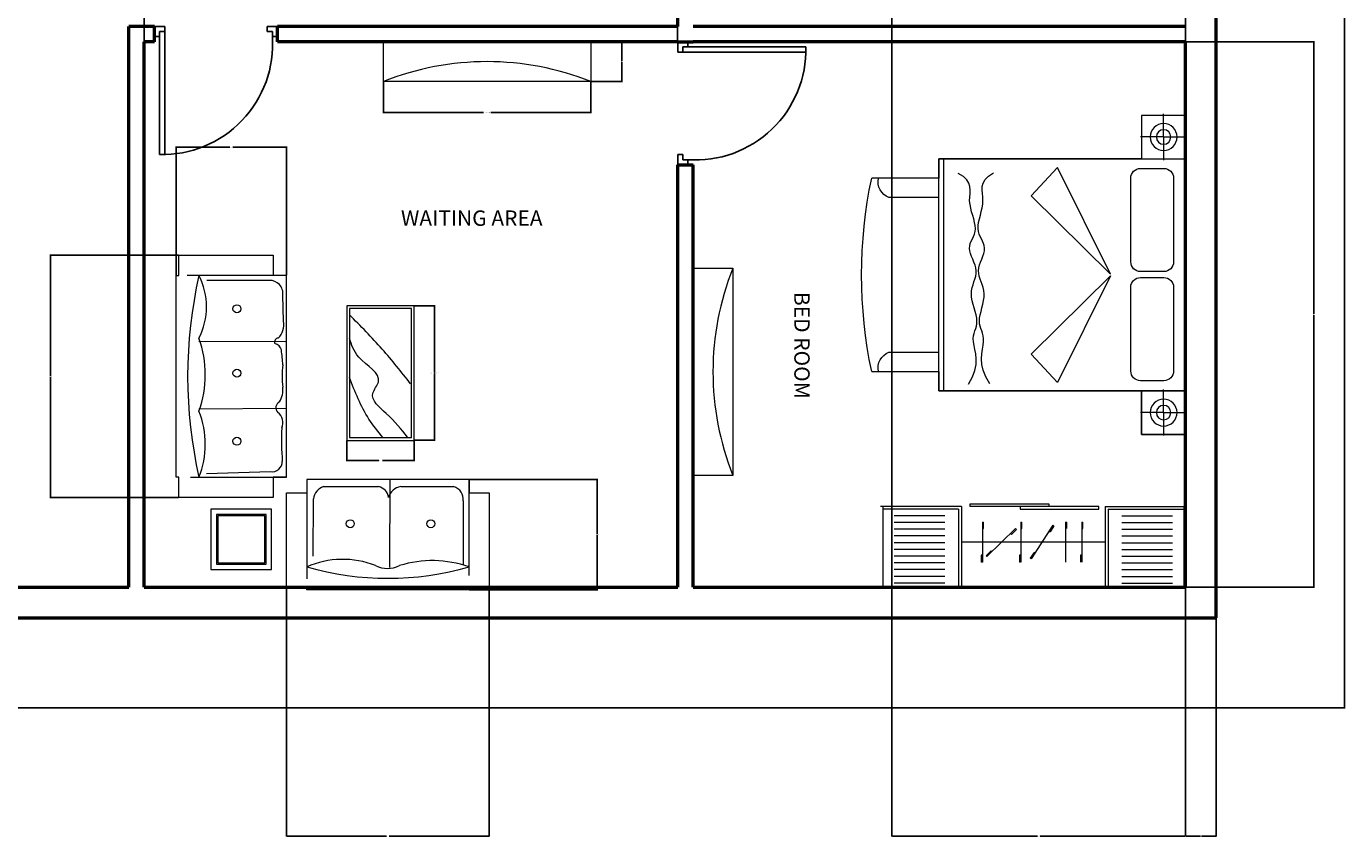
# Model space of a CAD drawing. Units: inches. Extents: x 1865 to 2541, y 1997 to 2759.
# Tile 3 of 11: x 2155 to 2541, y 1997 to 2234. Entities that reach past the tile are written whole.
import ezdxf

# ---------------------------------------------------------------- set-up
doc = ezdxf.new("R2010")
doc.units = ezdxf.units.IN
for name, color, linetype, lineweight in [('A-ANNO-DIMS', 2, 'Continuous', 18), ('A-AREA-IDEN', 4, 'Continuous', 18), ('A-FURN', 8, 'Continuous', 13), ('A-WALL', 7, 'Continuous', 50), ('BED', 42, 'Continuous', 13), ('CUPBOARD', 61, 'Continuous', 18), ('DOOR', 1, 'Continuous', 25), ('TV', 3, 'Continuous', 18)]:
    doc.layers.add(name, color=color, linetype=linetype, lineweight=lineweight)
doc.styles.get("Standard").update_dxf_attribs({"font": 'arial.ttf'})
doc.dimstyles.get("Standard").update_dxf_attribs({"dimtxt": 0.18, "dimasz": 0.18, "dimexe": 0.18, "dimexo": 0.0625, "dimgap": 0.09, "dimtad": 0, "dimtih": 1, "dimtoh": 1, "dimdec": 4, "dimzin": 0, "dimdsep": 46, "dimtxsty": 'Standard', "dimcen": 0.09, "dimadec": 0, "dimazin": 0, "dimtfac": 1, "dimtdec": 4, "dimtofl": 0, "dimtmove": 0, "dimatfit": 3, "dimfxl": 1, "dimtolj": 1, "dimtzin": 0, "dimarcsym": 0})

# ---------------------------------------------------------------- blocks, each defined once
blk = doc.blocks.new('A$C4F543DC7')
for p, q in [((0.013, 3.35, -0.169), (3.313, 3.35, -0.169)), ((0.463, 3.35, -0.169), (0.013, 3.35, -0.169)), ((0.013, 2.896, -0.169), (0.013, 3.35, -0.169)), ((0.013, 3.35, -0.169), (0.013, 2.896, -0.169)), ((0.238, 3.123, -0.439), (0.238, 3.361, -0.439)), ((0.463, 3.35, -0.169), (0.463, 0.8, -0.169)), ((2.863, 3.35, -0.169), (0.463, 3.35, -0.169)), ((0.463, 2.896, -0.169), (0.463, 3.35, -0.169)), ((2.863, 0.8, -0.169), (2.863, 3.35, -0.169)), ((2.863, 3.35, -0.169), (3.313, 3.35, -0.169)), ((2.863, 2.896, -0.169), (2.863, 3.35, -0.169)), ((3.089, 3.123, -0.439), (3.089, 3.361, -0.439)), ((3.313, 3.35, -0.169), (3.313, 2.896, -0.169)), ((3.313, 3.35, -0.169), (3.313, 2.896, -0.169)), ((1.535, 3.226, -0.169), (0.668, 3.226, -0.169)), ((2.664, 3.226, -0.169), (1.797, 3.226, -0.169)), ((0.238, 3.123, -0.439), (0, 3.123, -0.439)), ((0.238, 3.123, -0.439), (0.476, 3.123, -0.439)), ((0.238, 3.123, -0.439), (0.238, 2.885, -0.439)), ((0.568, 3.126, -0.169), (0.568, 2.884, -0.169)), ((1.635, 2.884, -0.169), (1.635, 3.126, -0.169)), ((1.697, 3.126, -0.169), (1.697, 2.884, -0.169)), ((2.764, 2.884, -0.169), (2.764, 3.126, -0.169)), ((3.089, 3.123, -0.439), (2.851, 3.123, -0.439)), ((3.089, 3.123, -0.439), (3.089, 2.885, -0.439)), ((3.089, 3.123, -0.439), (3.327, 3.123, -0.439)), ((0.463, 2.896, -0.169), (0.013, 2.896, -0.169)), ((0.013, 2.896, -0.169), (0.463, 2.896, -0.169)), ((0.463, 0.8, -0.169), (0.463, 2.896, -0.169)), ((2.863, 2.896, -0.169), (2.863, 0.8, -0.169)), ((3.313, 2.896, -0.169), (2.863, 2.896, -0.169)), ((3.313, 2.896, -0.169), (2.863, 2.896, -0.169)), ((0.668, 2.784, -0.169), (1.535, 2.784, -0.169)), ((1.797, 2.784, -0.169), (2.664, 2.784, -0.169)), ((1.653, 2.573, -0.169), (0.55, 2.025, -0.169)), ((0.841, 1.752, -0.169), (1.653, 2.573, -0.169)), ((2.481, 1.752, -0.169), (1.669, 2.573, -0.169)), ((1.669, 2.573, -0.169), (2.772, 2.025, -0.169)), ((0.55, 2.025, -0.169), (0.841, 1.752, -0.169)), ((2.772, 2.025, -0.169), (2.481, 1.752, -0.169)), ((0.537, 1.327, -0.169), (0.609, 1.284, -0.169)), ((0.609, 1.284, -0.169), (0.676, 1.257, -0.169)), ((0.676, 1.257, -0.169), (0.737, 1.243, -0.169)), ((0.737, 1.243, -0.169), (0.794, 1.239, -0.169)), ((0.794, 1.239, -0.169), (0.846, 1.242, -0.169)), ((0.846, 1.242, -0.169), (0.893, 1.249, -0.169)), ((0.893, 1.249, -0.169), (0.935, 1.256, -0.169)), ((0.935, 1.256, -0.169), (0.972, 1.261, -0.169)), ((0.972, 1.261, -0.169), (1.004, 1.262, -0.169)), ((1.004, 1.262, -0.169), (1.033, 1.258, -0.169)), ((1.033, 1.258, -0.169), (1.06, 1.251, -0.169)), ((1.06, 1.251, -0.169), (1.084, 1.242, -0.169)), ((1.084, 1.242, -0.169), (1.108, 1.234, -0.169)), ((1.108, 1.234, -0.169), (1.132, 1.226, -0.169)), ((1.25, 1.226, -0.169), (1.285, 1.235, -0.169)), ((1.285, 1.235, -0.169), (1.322, 1.244, -0.169)), ((1.322, 1.244, -0.169), (1.359, 1.253, -0.169)), ((1.359, 1.253, -0.169), (1.396, 1.261, -0.169)), ((1.396, 1.261, -0.169), (1.433, 1.266, -0.169)), ((1.433, 1.266, -0.169), (1.468, 1.268, -0.169)), ((1.468, 1.268, -0.169), (1.501, 1.264, -0.169)), ((1.501, 1.264, -0.169), (1.532, 1.257, -0.169)), ((1.532, 1.257, -0.169), (1.562, 1.247, -0.169)), ((1.562, 1.247, -0.169), (1.591, 1.237, -0.169)), ((1.591, 1.237, -0.169), (1.62, 1.226, -0.169)), ((1.765, 1.22, -0.169), (1.795, 1.23, -0.169)), ((1.795, 1.23, -0.169), (1.826, 1.242, -0.169)), ((1.826, 1.242, -0.169), (1.856, 1.253, -0.169)), ((1.856, 1.253, -0.169), (1.885, 1.263, -0.169)), ((1.885, 1.263, -0.169), (1.913, 1.27, -0.169)), ((1.913, 1.27, -0.169), (1.94, 1.272, -0.169)), ((1.94, 1.272, -0.169), (1.965, 1.269, -0.169)), ((1.965, 1.269, -0.169), (1.989, 1.262, -0.169)), ((1.989, 1.262, -0.169), (2.012, 1.251, -0.169)), ((2.012, 1.251, -0.169), (2.036, 1.239, -0.169)), ((2.036, 1.239, -0.169), (2.06, 1.227, -0.169)), ((2.279, 1.228, -0.169), (2.317, 1.238, -0.169)), ((2.317, 1.238, -0.169), (2.356, 1.246, -0.169)), ((2.356, 1.246, -0.169), (2.394, 1.253, -0.169)), ((2.394, 1.253, -0.169), (2.433, 1.255, -0.169)), ((2.433, 1.255, -0.169), (2.47, 1.253, -0.169)), ((2.47, 1.253, -0.169), (2.506, 1.249, -0.169)), ((2.506, 1.249, -0.169), (2.542, 1.246, -0.169)), ((2.542, 1.246, -0.169), (2.578, 1.248, -0.169)), ((2.578, 1.248, -0.169), (2.613, 1.257, -0.169)), ((2.613, 1.257, -0.169), (2.648, 1.277, -0.169)), ((2.648, 1.277, -0.169), (2.683, 1.312, -0.169)), ((2.683, 1.312, -0.169), (2.718, 1.364, -0.169)), ((0.533, 1.105, -0.169), (0.607, 1.146, -0.169)), ((0.607, 1.146, -0.169), (0.674, 1.171, -0.169)), ((0.674, 1.171, -0.169), (0.736, 1.183, -0.169)), ((0.736, 1.183, -0.169), (0.793, 1.185, -0.169)), ((0.793, 1.185, -0.169), (0.845, 1.18, -0.169)), ((0.845, 1.18, -0.169), (0.891, 1.172, -0.169)), ((0.891, 1.172, -0.169), (0.933, 1.163, -0.169)), ((0.933, 1.163, -0.169), (0.97, 1.156, -0.169)), ((0.97, 1.156, -0.169), (1.003, 1.155, -0.169)), ((1.003, 1.155, -0.169), (1.032, 1.158, -0.169)), ((1.032, 1.158, -0.169), (1.058, 1.164, -0.169)), ((1.058, 1.164, -0.169), (1.083, 1.172, -0.169)), ((1.083, 1.172, -0.169), (1.107, 1.18, -0.169)), ((1.107, 1.18, -0.169), (1.132, 1.187, -0.169)), ((1.132, 1.226, -0.169), (1.158, 1.22, -0.169)), ((1.132, 1.187, -0.169), (1.157, 1.192, -0.169)), ((1.157, 1.192, -0.169), (1.185, 1.193, -0.169)), ((1.158, 1.22, -0.169), (1.185, 1.218, -0.169)), ((1.185, 1.218, -0.169), (1.216, 1.22, -0.169)), ((1.185, 1.193, -0.169), (1.216, 1.19, -0.169)), ((1.216, 1.22, -0.169), (1.25, 1.226, -0.169)), ((1.216, 1.19, -0.169), (1.249, 1.183, -0.169)), ((1.249, 1.183, -0.169), (1.284, 1.173, -0.169)), ((1.284, 1.173, -0.169), (1.321, 1.163, -0.169)), ((1.321, 1.163, -0.169), (1.358, 1.152, -0.169)), ((1.358, 1.152, -0.169), (1.394, 1.143, -0.169)), ((1.394, 1.143, -0.169), (1.431, 1.137, -0.169)), ((1.431, 1.137, -0.169), (1.466, 1.135, -0.169)), ((1.466, 1.135, -0.169), (1.499, 1.137, -0.169)), ((1.499, 1.137, -0.169), (1.531, 1.143, -0.169)), ((1.531, 1.143, -0.169), (1.561, 1.152, -0.169)), ((1.561, 1.152, -0.169), (1.59, 1.162, -0.169)), ((1.59, 1.162, -0.169), (1.619, 1.172, -0.169)), ((1.619, 1.172, -0.169), (1.648, 1.18, -0.169)), ((1.62, 1.226, -0.169), (1.648, 1.217, -0.169)), ((1.648, 1.217, -0.169), (1.676, 1.211, -0.169)), ((1.648, 1.18, -0.169), (1.676, 1.185, -0.169)), ((1.676, 1.211, -0.169), (1.705, 1.209, -0.169)), ((1.676, 1.185, -0.169), (1.705, 1.186, -0.169)), ((1.705, 1.209, -0.169), (1.735, 1.212, -0.169)), ((1.705, 1.186, -0.169), (1.734, 1.182, -0.169)), ((1.734, 1.182, -0.169), (1.764, 1.173, -0.169)), ((1.735, 1.212, -0.169), (1.765, 1.22, -0.169)), ((1.764, 1.173, -0.169), (1.794, 1.162, -0.169)), ((1.794, 1.162, -0.169), (1.824, 1.149, -0.169)), ((1.824, 1.149, -0.169), (1.854, 1.137, -0.169)), ((1.854, 1.137, -0.169), (1.883, 1.126, -0.169)), ((1.883, 1.126, -0.169), (1.911, 1.119, -0.169)), ((1.911, 1.119, -0.169), (1.937, 1.115, -0.169)), ((1.937, 1.115, -0.169), (1.963, 1.118, -0.169)), ((1.963, 1.118, -0.169), (1.987, 1.124, -0.169)), ((1.987, 1.124, -0.169), (2.011, 1.134, -0.169)), ((2.011, 1.134, -0.169), (2.034, 1.145, -0.169)), ((2.034, 1.145, -0.169), (2.059, 1.157, -0.169)), ((2.059, 1.157, -0.169), (2.084, 1.167, -0.169)), ((2.06, 1.227, -0.169), (2.085, 1.216, -0.169)), ((2.084, 1.167, -0.169), (2.111, 1.174, -0.169)), ((2.085, 1.216, -0.169), (2.112, 1.208, -0.169)), ((2.111, 1.174, -0.169), (2.14, 1.177, -0.169)), ((2.112, 1.208, -0.169), (2.141, 1.204, -0.169)), ((2.14, 1.177, -0.169), (2.172, 1.175, -0.169)), ((2.141, 1.204, -0.169), (2.172, 1.205, -0.169)), ((2.172, 1.205, -0.169), (2.206, 1.21, -0.169)), ((2.172, 1.175, -0.169), (2.206, 1.169, -0.169)), ((2.206, 1.21, -0.169), (2.242, 1.218, -0.169)), ((2.206, 1.169, -0.169), (2.241, 1.16, -0.169)), ((2.241, 1.16, -0.169), (2.278, 1.149, -0.169)), ((2.242, 1.218, -0.169), (2.279, 1.228, -0.169)), ((2.278, 1.149, -0.169), (2.316, 1.138, -0.169)), ((2.316, 1.138, -0.169), (2.354, 1.128, -0.169)), ((2.354, 1.128, -0.169), (2.392, 1.121, -0.169)), ((2.392, 1.121, -0.169), (2.43, 1.117, -0.169)), ((2.43, 1.117, -0.169), (2.468, 1.118, -0.169)), ((2.468, 1.118, -0.169), (2.504, 1.121, -0.169)), ((2.504, 1.121, -0.169), (2.54, 1.123, -0.169)), ((2.54, 1.123, -0.169), (2.576, 1.12, -0.169)), ((2.576, 1.12, -0.169), (2.611, 1.109, -0.169)), ((2.611, 1.109, -0.169), (2.645, 1.088, -0.169)), ((2.645, 1.088, -0.169), (2.679, 1.052, -0.169)), ((2.679, 1.052, -0.169), (2.712, 0.999, -0.169)), ((0.463, 0.85, -0.169), (2.863, 0.85, -0.169)), ((0.463, 0.8, -0.169), (2.863, 0.8, -0.169)), ((0.663, 0.8, -0.169), (0.463, 0.8, -0.169)), ((0.663, 0.8, -0.169), (2.663, 0.8, -0.169)), ((0.663, 0.104, -0.169), (0.663, 0.8, -0.169)), ((0.663, 0.104, -0.169), (0.663, 0.8, -0.169)), ((0.863, 0.281, -0.169), (0.863, 0.8, -0.169)), ((2.463, 0.8, -0.169), (2.463, 0.281, -0.169)), ((2.863, 0.8, -0.169), (2.663, 0.8, -0.169)), ((2.663, 0.8, -0.169), (2.663, 0.104, -0.169)), ((2.663, 0.8, -0.169), (2.663, 0.104, -0.169))]:
    blk.add_line(p, q)
for centre, radius in [((0.238, 3.123, -0.439), 0.139), ((0.238, 3.123, -0.439), 0.075), ((3.089, 3.123, -0.439), 0.139), ((3.089, 3.123, -0.439), 0.075)]:
    blk.add_circle(centre, radius)
for centre, radius, start, end in [((0.668, 3.126, -0.169), 0.1, 90, 180), ((1.535, 3.126, -0.169), 0.1, 0, 90), ((1.797, 3.126, -0.169), 0.1, 90, 180), ((2.664, 3.126, -0.169), 0.1, 0, 90), ((0.668, 2.884, -0.169), 0.1, 180, 270), ((1.535, 2.884, -0.169), 0.1, 270, 0), ((1.797, 2.884, -0.169), 0.1, 180, 270), ((2.664, 2.884, -0.169), 0.1, 270, 0), ((0.699, 0.347, -0.169), 0.177, 258.2616, 338.032), ((2.627, 0.347, -0.169), 0.177, 201.968, 281.7384), ((1.663, 4.86, -0.169), 4.86, 258.1252, 281.8748), ((1.663, 4.86, -0.169), 4.86, 258.1252, 281.8748)]:
    blk.add_arc(centre, radius, start, end)
blk = doc.blocks.new('A$C34930FF8')
for p, q in [((600, 1669.3), (600, 2269.3)), ((30, 1790.9), (30, 2169.3)), ((80, 1790.9), (80, 2169.3)), ((130, 1790.9), (130, 2169.3)), ((180, 1790.9), (180, 2169.3)), ((230, 1790.9), (230, 2169.3)), ((280, 1790.9), (280, 2169.3)), ((330, 1790.9), (330, 2169.3)), ((380, 1790.9), (380, 2169.3)), ((430, 1790.9), (430, 2169.3)), ((480, 1790.9), (480, 2169.3)), ((530, 1790.9), (530, 2169.3)), ((580, 1690.9), (580, 2252.4)), ((580, 1690.9), (0, 1690.9)), ((600, 1669.3), (0, 1669.3)), ((335.4, 1666.1), (335.4, 603.1)), ((600, 1603.3), (620, 1603.3)), ((600, 1018.7), (600, 1603.3)), ((620, 1603.3), (620, 1018.7)), ((237.7, 1521.5), (185.4, 1521.5)), ((482.5, 1513), (185.4, 1513)), ((434.8, 1266.1), (227.4, 1478.9)), ((269.7, 1447.7), (233.2, 1485.2)), ((436.7, 1504.4), (482.5, 1504.4)), ((428.7, 1260.1), (392.1, 1297.6)), ((237.7, 1237.7), (185.4, 1237.7)), ((482.5, 1228.2), (185.4, 1228.2)), ((436.7, 1219.7), (482.5, 1219.7)), ((600, 1233.4), (580, 1233.4)), ((580, 1233.4), (580, 648.7)), ((600, 648.7), (600, 1233.4)), ((459.3, 989.3), (209.5, 1150.1)), ((258.1, 1129), (214.1, 1157.3)), ((454.7, 982.1), (410.6, 1010.5)), ((620, 1018.7), (600, 1018.7)), ((482.5, 894.9), (185.4, 894.9)), ((436.7, 886.3), (482.5, 886.3)), ((237.7, 783.9), (185.4, 783.9)), ((482.5, 775.3), (185.4, 775.3)), ((436.7, 766.8), (482.5, 766.8)), ((600, 600), (0, 600)), ((580, 648.7), (600, 648.7)), ((600, 600), (600, 0)), ((580, 578.3), (0, 578.3)), ((580, 578.3), (580, 16.8)), ((30, 478.3), (30, 100)), ((80, 478.3), (80, 100)), ((130, 478.3), (130, 100)), ((180, 478.3), (180, 100)), ((230, 478.3), (230, 100)), ((280, 478.3), (280, 100)), ((330, 478.3), (330, 100)), ((380, 478.3), (380, 100)), ((430, 478.3), (430, 100)), ((480, 478.3), (480, 100)), ((530, 478.3), (530, 100))]:
    blk.add_line(p, q)
at = {"ltscale": 0.05}
for p, q in [((0, 2252.4), (0, 16.8)), ((600, 2252.4), (0, 2252.4)), ((185.4, 1513), (185.4, 1521.5)), ((227.1, 1479.2), (233.2, 1485.2)), ((237.7, 1513), (237.7, 1521.5)), ((436.7, 1513), (436.7, 1504.4)), ((482.5, 1513), (482.5, 1504.4)), ((263.6, 1441.7), (269.7, 1447.7)), ((398.2, 1303.6), (392.1, 1297.6)), ((185.4, 1229.1), (185.4, 1237.7)), ((237.7, 1229.1), (237.7, 1237.7)), ((434.8, 1266.1), (428.7, 1260.1)), ((436.7, 1228.2), (436.7, 1219.7)), ((482.5, 1228.2), (482.5, 1219.7)), ((209.5, 1150.1), (214.1, 1157.3)), ((253.5, 1121.8), (258.1, 1129)), ((415.3, 1017.6), (410.6, 1010.5)), ((459.3, 989.3), (454.7, 982.1)), ((482.5, 894.9), (482.5, 886.3)), ((237.7, 775.3), (237.7, 783.9)), ((436.7, 775.3), (436.7, 766.8)), ((482.5, 775.3), (482.5, 766.8)), ((600, 16.8), (0, 16.8))]:
    blk.add_line(p, q, dxfattribs=at)
blk = doc.blocks.new('DOOR-SWING-36IN')
for p, q in [((34.51, 36), (37.51, 36)), ((34.51, 34.5), (34.51, 36)), ((37.51, 36), (37.51, 33)), ((36.01, 34.5), (0.01, 34.5)), ((36.01, 33), (0.01, 33)), ((36.01, 34.5), (34.51, 34.5)), ((36.01, 33), (36.01, 34.5)), ((37.51, 33), (36.01, 33)), ((36.01, 1.5), (34.51, 1.5)), ((34.51, 1.5), (34.51, 0)), ((34.51, 0), (37.51, 0)), ((37.51, 3), (36.01, 3)), ((36.01, 3), (36.01, 1.5)), ((37.51, 0), (37.51, 3))]:
    blk.add_line(p, q)
blk.add_arc((32.32, 33.75), 32.32, 178.6705, 273.8756)
blk = doc.blocks.new('TABLE-COFFEE-RECT')
for p, q in [((0, 39.37), (0, 0)), ((19.69, 39.37), (0, 39.37)), ((0.79, 38.58), (0.79, 0.79)), ((18.9, 38.58), (0.79, 38.58)), ((18.9, 0.79), (18.9, 38.58)), ((19.69, 0), (19.69, 39.37)), ((0.79, 0.79), (18.9, 0.79)), ((0, 0), (19.69, 0))]:
    blk.add_line(p, q)
for points, knots in [([(18.6, 16.56), (15.9, 19.98), (10.33, 27.05), (3.98, 33.45), (0.7, 36.75)], [0, 0, 0, 0, 13.044093, 27.000677, 27.000677, 27.000677, 27.000677]), ([(17.68, 0.96), (15.88, 3.19), (12.68, 7.14), (5.8, 12.67), (11.59, 18.88), (2.91, 23.18), (1.33, 27.96), (0.7, 29.87)], [0, 0, 0, 0, 9.260592, 16.388167, 19.979545, 29.29681, 35.453459, 35.453459, 35.453459, 35.453459]), ([(10.57, 0.73), (9.12, 2.52), (4.86, 7.82), (2.36, 14.19), (0.7, 18.4)], [0, 0, 0, 0, 6.883342, 20.328879, 20.328879, 20.328879, 20.328879])]:
    blk.add_open_spline(points, degree=3, knots=knots)
blk = doc.blocks.new('TV-UNIT')
blk.add_lwpolyline([(0, 11.62), (60.65, 11.62), (60.65, 0), (0, 0)], close=True)
blk.add_arc((30.32, -76.26), 82.06, 68.3146, 111.6854)
blk = doc.blocks.new('*D22')
at = {"layer": 'A-ANNO-DIMS', "color": 0, "lineweight": -2, "transparency": 16777216}
for p, q in [((2259.69, 2218.27), (2259.69, 2209.06)), ((2320.34, 2218.27), (2320.34, 2209.06)), ((2259.87, 2209.24), (2288.96, 2209.24)), ((2320.16, 2209.24), (2291.07, 2209.24))]:
    blk.add_line(p, q, dxfattribs=at)
at = {"layer": 'A-ANNO-DIMS', "color": 0, "transparency": 16777216}
for points in [[(2259.87, 2209.27), (2259.87, 2209.21), (2259.69, 2209.24)], [(2320.16, 2209.27), (2320.16, 2209.21), (2320.34, 2209.24)]]:
    blk.add_solid(points, dxfattribs=at)
at = {"layer": 'Defpoints', "color": 0, "transparency": 16777216}
for p in [(2259.69, 2218.33), (2320.34, 2218.33), (2320.34, 2209.24)]:
    blk.add_point(p, dxfattribs=at)
at = {"layer": 'A-ANNO-DIMS', "color": 0, "transparency": 16777216, "insert": (2290.02, 2209.24), "char_height": 0.18, "attachment_point": 5}
blk.add_mtext('\\A1;TV UNIT 61 TYP.', dxfattribs=at)
blk = doc.blocks.new('*D23')
at = {"layer": 'A-ANNO-DIMS', "color": 0, "lineweight": -2, "transparency": 16777216}
for p, q in [((2320.4, 2229.95), (2329.62, 2229.95)), ((2329.44, 2229.77), (2329.44, 2224.32)), ((2329.44, 2218.51), (2329.44, 2223.96)), ((2320.4, 2218.33), (2329.62, 2218.33))]:
    blk.add_line(p, q, dxfattribs=at)
at = {"layer": 'A-ANNO-DIMS', "color": 0, "transparency": 16777216}
for points in [[(2329.41, 2229.77), (2329.47, 2229.77), (2329.44, 2229.95)], [(2329.41, 2218.51), (2329.47, 2218.51), (2329.44, 2218.33)]]:
    blk.add_solid(points, dxfattribs=at)
at = {"layer": 'Defpoints', "color": 0, "transparency": 16777216}
for p in [(2320.34, 2229.95), (2329.44, 2229.95), (2320.34, 2218.33)]:
    blk.add_point(p, dxfattribs=at)
at = {"layer": 'A-ANNO-DIMS', "color": 0, "transparency": 16777216, "insert": (2329.44, 2224.14), "char_height": 0.18, "attachment_point": 5}
blk.add_mtext('\\A1;12 TYP.', dxfattribs=at)
blk = doc.blocks.new('*D36')
at = {"layer": 'A-ANNO-DIMS', "color": 0, "lineweight": -2, "transparency": 16777216}
for p, q in [((2268.79, 2152.76), (2274.81, 2152.76)), ((2274.63, 2152.58), (2274.63, 2133.25)), ((2274.63, 2113.57), (2274.63, 2132.89)), ((2268.79, 2113.39), (2274.81, 2113.39))]:
    blk.add_line(p, q, dxfattribs=at)
at = {"layer": 'A-ANNO-DIMS', "color": 0, "transparency": 16777216}
for points in [[(2274.6, 2152.58), (2274.66, 2152.58), (2274.63, 2152.76)], [(2274.6, 2113.57), (2274.66, 2113.57), (2274.63, 2113.39)]]:
    blk.add_solid(points, dxfattribs=at)
at = {"layer": 'Defpoints', "color": 0, "transparency": 16777216}
for p in [(2268.73, 2152.76), (2274.63, 2152.76), (2268.73, 2113.39)]:
    blk.add_point(p, dxfattribs=at)
at = {"layer": 'A-ANNO-DIMS', "color": 0, "transparency": 16777216, "insert": (2274.63, 2133.07), "char_height": 0.18, "attachment_point": 5}
blk.add_mtext('\\A1;COFFEE TABLE 39 TYP.', dxfattribs=at)
blk = doc.blocks.new('*D37')
at = {"layer": 'A-ANNO-DIMS', "color": 0, "lineweight": -2, "transparency": 16777216}
for p, q in [((2249.04, 2113.32), (2249.04, 2107.3)), ((2268.73, 2113.32), (2268.73, 2107.3)), ((2249.22, 2107.48), (2258.35, 2107.48)), ((2268.55, 2107.48), (2259.41, 2107.48))]:
    blk.add_line(p, q, dxfattribs=at)
at = {"layer": 'A-ANNO-DIMS', "color": 0, "transparency": 16777216}
for points in [[(2249.22, 2107.51), (2249.22, 2107.45), (2249.04, 2107.48)], [(2268.55, 2107.51), (2268.55, 2107.45), (2268.73, 2107.48)]]:
    blk.add_solid(points, dxfattribs=at)
at = {"layer": 'Defpoints', "color": 0, "transparency": 16777216}
for p in [(2249.04, 2113.39), (2268.73, 2113.39), (2268.73, 2107.48)]:
    blk.add_point(p, dxfattribs=at)
at = {"layer": 'A-ANNO-DIMS', "color": 0, "transparency": 16777216, "insert": (2258.88, 2107.48), "char_height": 0.18, "attachment_point": 5}
blk.add_mtext('\\A1;20 TYP.', dxfattribs=at)
blk = doc.blocks.new('*D41')
at = {"layer": 'A-ANNO-DIMS', "color": 0, "lineweight": -2, "transparency": 16777216}
for p, q in [((2503.31, 2721.45), (2540.92, 2721.45)), ((2540.74, 2721.27), (2540.74, 2378.49)), ((2540.74, 2035.35), (2540.74, 2378.13)), ((2136.19, 2035.17), (2540.92, 2035.17))]:
    blk.add_line(p, q, dxfattribs=at)
at = {"layer": 'A-ANNO-DIMS', "color": 0, "transparency": 16777216}
for points in [[(2540.71, 2721.27), (2540.77, 2721.27), (2540.74, 2721.45)], [(2540.71, 2035.35), (2540.77, 2035.35), (2540.74, 2035.17)]]:
    blk.add_solid(points, dxfattribs=at)
at = {"layer": 'Defpoints', "color": 0, "transparency": 16777216}
for p in [(2503.24, 2721.45), (2136.13, 2035.17), (2540.74, 2035.17)]:
    blk.add_point(p, dxfattribs=at)
at = {"layer": 'A-ANNO-DIMS', "color": 0, "transparency": 16777216, "insert": (2540.74, 2378.31), "char_height": 0.18, "attachment_point": 5}
blk.add_mtext('\\A1;686.3', dxfattribs=at)
blk = doc.blocks.new('*D54')
at = {"layer": 'A-ANNO-DIMS', "color": 0, "lineweight": -2, "transparency": 16777216}
for p, q in [((2189.74, 2230.01), (2189.74, 2267.63)), ((2189.92, 2267.45), (2267.46, 2267.45)), ((2345.56, 2267.45), (2268.02, 2267.45)), ((2345.74, 2230.01), (2345.74, 2267.63))]:
    blk.add_line(p, q, dxfattribs=at)
at = {"layer": 'A-ANNO-DIMS', "color": 0, "transparency": 16777216}
for points in [[(2189.92, 2267.48), (2189.92, 2267.42), (2189.74, 2267.45)], [(2345.56, 2267.48), (2345.56, 2267.42), (2345.74, 2267.45)]]:
    blk.add_solid(points, dxfattribs=at)
at = {"layer": 'Defpoints', "color": 0, "transparency": 16777216}
for p in [(2345.74, 2267.45), (2189.74, 2229.95), (2345.74, 2229.95)]:
    blk.add_point(p, dxfattribs=at)
at = {"layer": 'A-ANNO-DIMS', "color": 0, "transparency": 16777216, "insert": (2267.74, 2267.45), "char_height": 0.18, "attachment_point": 5}
blk.add_mtext('\\A1;156', dxfattribs=at)
blk = doc.blocks.new('*D55')
at = {"layer": 'A-ANNO-DIMS', "color": 0, "lineweight": -2, "transparency": 16777216}
for p, q in [((2494.31, 2229.95), (2531.92, 2229.95)), ((2531.74, 2229.77), (2531.74, 2150.38)), ((2531.74, 2070.63), (2531.74, 2150.02)), ((2494.31, 2070.45), (2531.92, 2070.45))]:
    blk.add_line(p, q, dxfattribs=at)
at = {"layer": 'A-ANNO-DIMS', "color": 0, "transparency": 16777216}
for points in [[(2531.71, 2229.77), (2531.77, 2229.77), (2531.74, 2229.95)], [(2531.71, 2070.63), (2531.77, 2070.63), (2531.74, 2070.45)]]:
    blk.add_solid(points, dxfattribs=at)
at = {"layer": 'Defpoints', "color": 0, "transparency": 16777216}
for p in [(2494.24, 2229.95), (2494.24, 2070.45), (2531.74, 2070.45)]:
    blk.add_point(p, dxfattribs=at)
at = {"layer": 'A-ANNO-DIMS', "color": 0, "transparency": 16777216, "insert": (2531.74, 2150.2), "char_height": 0.18, "attachment_point": 5}
blk.add_mtext('\\A1;159.5', dxfattribs=at)
blk = doc.blocks.new('*D59')
at = {"layer": 'A-ANNO-DIMS', "color": 0, "lineweight": -2, "transparency": 16777216}
for p, q in [((2494.24, 2070.39), (2494.24, 1997.49)), ((2503.24, 2061.39), (2503.24, 1997.49)), ((2494.42, 1997.67), (2498.59, 1997.67)), ((2503.06, 1997.67), (2498.89, 1997.67))]:
    blk.add_line(p, q, dxfattribs=at)
at = {"layer": 'A-ANNO-DIMS', "color": 0, "transparency": 16777216}
for points in [[(2494.42, 1997.7), (2494.42, 1997.64), (2494.24, 1997.67)], [(2503.06, 1997.7), (2503.06, 1997.64), (2503.24, 1997.67)]]:
    blk.add_solid(points, dxfattribs=at)
at = {"layer": 'Defpoints', "color": 0, "transparency": 16777216}
for p in [(2494.24, 2070.45), (2503.24, 2061.45), (2503.24, 1997.67)]:
    blk.add_point(p, dxfattribs=at)
at = {"layer": 'A-ANNO-DIMS', "color": 0, "transparency": 16777216, "insert": (2498.74, 1997.67), "char_height": 0.18, "attachment_point": 5}
blk.add_mtext('\\A1;9', dxfattribs=at)
blk = doc.blocks.new('*D64')
at = {"layer": 'A-ANNO-DIMS', "color": 0, "lineweight": -2, "transparency": 16777216}
for p, q in [((2408.38, 2406.89), (2408.38, 1997.49)), ((2494.24, 2406.89), (2494.24, 1997.49)), ((2408.56, 1997.67), (2450.92, 1997.67)), ((2494.06, 1997.67), (2451.7, 1997.67))]:
    blk.add_line(p, q, dxfattribs=at)
at = {"layer": 'A-ANNO-DIMS', "color": 0, "transparency": 16777216}
for points in [[(2408.56, 1997.7), (2408.56, 1997.64), (2408.38, 1997.67)], [(2494.06, 1997.7), (2494.06, 1997.64), (2494.24, 1997.67)]]:
    blk.add_solid(points, dxfattribs=at)
at = {"layer": 'Defpoints', "color": 0, "transparency": 16777216}
for p in [(2408.38, 2406.95), (2494.24, 2406.95), (2494.24, 1997.67)]:
    blk.add_point(p, dxfattribs=at)
at = {"layer": 'A-ANNO-DIMS', "color": 0, "transparency": 16777216, "insert": (2451.31, 1997.67), "char_height": 0.18, "attachment_point": 5}
blk.add_mtext('\\A1;85.87', dxfattribs=at)
blk = doc.blocks.new('*D71')
at = {"layer": 'A-ANNO-DIMS', "color": 0, "lineweight": -2, "transparency": 16777216}
for p, q in [((2199.81, 2167.53), (2162.19, 2167.53)), ((2162.37, 2167.35), (2162.37, 2132.28)), ((2162.37, 2096.85), (2162.37, 2131.92)), ((2199.81, 2096.67), (2162.19, 2096.67))]:
    blk.add_line(p, q, dxfattribs=at)
at = {"layer": 'A-ANNO-DIMS', "color": 0, "transparency": 16777216}
for points in [[(2162.34, 2167.35), (2162.4, 2167.35), (2162.37, 2167.53)], [(2162.34, 2096.85), (2162.4, 2096.85), (2162.37, 2096.67)]]:
    blk.add_solid(points, dxfattribs=at)
at = {"layer": 'Defpoints', "color": 0, "transparency": 16777216}
for p in [(2162.37, 2167.53), (2199.87, 2167.53), (2199.87, 2096.67)]:
    blk.add_point(p, dxfattribs=at)
at = {"layer": 'A-ANNO-DIMS', "color": 0, "transparency": 16777216, "insert": (2162.37, 2132.1), "char_height": 0.18, "attachment_point": 5}
blk.add_mtext('\\A1;70.87', dxfattribs=at)
blk = doc.blocks.new('*D72')
at = {"layer": 'A-ANNO-DIMS', "color": 0, "lineweight": -2, "transparency": 16777216}
for p, q in [((2231.4, 2070.39), (2231.4, 1997.49)), ((2290.66, 2070.39), (2290.66, 1997.49)), ((2231.58, 1997.67), (2260.63, 1997.67)), ((2290.48, 1997.67), (2261.42, 1997.67))]:
    blk.add_line(p, q, dxfattribs=at)
at = {"layer": 'A-ANNO-DIMS', "color": 0, "transparency": 16777216}
for points in [[(2231.58, 1997.7), (2231.58, 1997.64), (2231.4, 1997.67)], [(2290.48, 1997.7), (2290.48, 1997.64), (2290.66, 1997.67)]]:
    blk.add_solid(points, dxfattribs=at)
at = {"layer": 'Defpoints', "color": 0, "transparency": 16777216}
for p in [(2231.4, 2070.45), (2290.66, 2070.45), (2290.66, 1997.67)]:
    blk.add_point(p, dxfattribs=at)
at = {"layer": 'A-ANNO-DIMS', "color": 0, "transparency": 16777216, "insert": (2261.03, 1997.67), "char_height": 0.18, "attachment_point": 5}
blk.add_mtext('\\A1;59.26', dxfattribs=at)
blk = doc.blocks.new('*D73')
at = {"layer": 'A-ANNO-DIMS', "color": 0, "lineweight": -2, "transparency": 16777216}
for p, q in [((2284.81, 2101.95), (2322.43, 2101.95)), ((2322.25, 2101.77), (2322.25, 2085.99)), ((2322.25, 2069.84), (2322.25, 2085.62)), ((2284.81, 2069.66), (2322.43, 2069.66))]:
    blk.add_line(p, q, dxfattribs=at)
at = {"layer": 'A-ANNO-DIMS', "color": 0, "transparency": 16777216}
for points in [[(2322.22, 2101.77), (2322.28, 2101.77), (2322.25, 2101.95)], [(2322.22, 2069.84), (2322.28, 2069.84), (2322.25, 2069.66)]]:
    blk.add_solid(points, dxfattribs=at)
at = {"layer": 'Defpoints', "color": 0, "transparency": 16777216}
for p in [(2284.75, 2101.95), (2284.75, 2069.66), (2322.25, 2069.66)]:
    blk.add_point(p, dxfattribs=at)
at = {"layer": 'A-ANNO-DIMS', "color": 0, "transparency": 16777216, "insert": (2322.25, 2085.8), "char_height": 0.18, "attachment_point": 5}
blk.add_mtext('\\A1;32.283', dxfattribs=at)
blk = doc.blocks.new('*D74')
at = {"layer": 'A-ANNO-DIMS', "color": 0, "lineweight": -2, "transparency": 16777216}
for p, q in [((2199.08, 2161.69), (2199.08, 2199.31)), ((2199.26, 2199.13), (2214.76, 2199.13)), ((2231.19, 2199.13), (2215.69, 2199.13)), ((2231.37, 2161.69), (2231.37, 2199.31))]:
    blk.add_line(p, q, dxfattribs=at)
at = {"layer": 'A-ANNO-DIMS', "color": 0, "transparency": 16777216}
for points in [[(2199.26, 2199.16), (2199.26, 2199.1), (2199.08, 2199.13)], [(2231.19, 2199.16), (2231.19, 2199.1), (2231.37, 2199.13)]]:
    blk.add_solid(points, dxfattribs=at)
at = {"layer": 'Defpoints', "color": 0, "transparency": 16777216}
for p in [(2231.37, 2199.13), (2199.08, 2161.63), (2231.37, 2161.63)]:
    blk.add_point(p, dxfattribs=at)
at = {"layer": 'A-ANNO-DIMS', "color": 0, "transparency": 16777216, "insert": (2215.22, 2199.13), "char_height": 0.18, "attachment_point": 5}
blk.add_mtext('\\A1;32.283', dxfattribs=at)

msp = doc.modelspace()

# ---------------------------------------------------------------- linework, layer by layer
at = {"layer": 'A-FURN'}
for p, q in [((2199.8707, 2167.5338), (2227.4297, 2167.5338)), ((2199.8707, 2161.6283), (2199.8707, 2167.5338)), ((2227.4297, 2167.5338), (2227.4297, 2161.6283)), ((2199.0833, 2102.5732), (2199.0833, 2161.6283)), ((2199.0833, 2161.6283), (2199.8707, 2161.6283)), ((2231.3667, 2161.6283), (2202.2959, 2161.6283)), ((2226.3265, 2160.1618), (2208.0964, 2160.1618)), ((2231.3667, 2102.5732), (2231.3667, 2161.6283)), ((2230.4697, 2148.2092), (2230.304, 2155.8529)), ((2231.3667, 2142.2304), (2205.7762, 2142.3045)), ((2231.3667, 2122.6687), (2205.7762, 2122.5149)), ((2199.8707, 2102.5732), (2199.0833, 2102.5732)), ((2199.8707, 2096.6677), (2199.8707, 2102.5732)), ((2203.2903, 2102.5732), (2231.3667, 2102.5732)), ((2207.9307, 2103.7333), (2226.658, 2104.2305)), ((2231.3667, 2102.5732), (2227.4297, 2102.5732)), ((2227.4297, 2102.5732), (2227.4297, 2096.6677)), ((2284.7519, 2101.9455), (2237.3042, 2101.9455)), ((2237.3042, 2101.9455), (2237.3042, 2072.8746)), ((2242.1744, 2099.8408), (2258.2878, 2099.8408)), ((2261.5859, 2101.8186), (2261.5118, 2076.2281)), ((2264.7585, 2099.8408), (2280.2374, 2099.8408)), ((2284.7519, 2101.9455), (2284.7519, 2098.0085)), ((2284.7519, 2073.869), (2284.7519, 2101.9455)), ((2227.4297, 2096.6677), (2199.8707, 2096.6677)), ((2231.3987, 2098.0085), (2237.3042, 2098.0085)), ((2231.3987, 2070.4494), (2231.3987, 2098.0085)), ((2239.1294, 2079.5406), (2239.2563, 2096.2883)), ((2283.0287, 2095.6539), (2283.0287, 2076.8762)), ((2284.7519, 2098.0085), (2290.6574, 2098.0085)), ((2290.6574, 2098.0085), (2290.6574, 2070.4494)), ((2226.9931, 2093.2909), (2209.2765, 2093.2909)), ((2209.2765, 2093.2909), (2209.2765, 2075.5744)), ((2225.4183, 2091.7161), (2210.8513, 2091.7161)), ((2210.8513, 2091.7161), (2210.8513, 2077.1492)), ((2225.0246, 2091.3224), (2211.245, 2091.3224)), ((2211.245, 2091.3224), (2211.245, 2077.5429)), ((2225.0246, 2077.5429), (2225.0246, 2091.3224)), ((2225.4183, 2077.1492), (2225.4183, 2091.7161)), ((2226.9931, 2075.5744), (2226.9931, 2093.2909)), ((2209.2765, 2075.5744), (2226.9931, 2075.5744)), ((2210.8513, 2077.1492), (2225.4183, 2077.1492)), ((2211.245, 2077.5429), (2225.0246, 2077.5429)), ((2237.3042, 2070.4494), (2231.3987, 2070.4494)), ((2237.3042, 2069.662), (2237.3042, 2070.4494)), ((2284.7519, 2069.662), (2237.3042, 2069.662)), ((2284.7519, 2070.4494), (2284.7519, 2069.662)), ((2290.6574, 2070.4494), (2284.7519, 2070.4494))]:
    msp.add_line(p, q, dxfattribs=at)
for centre in [(2216.88, 2151.8561), (2216.88, 2133.0267), (2216.88, 2113.1307), (2249.9945, 2088.9813), (2273.56, 2088.9813)]:
    msp.add_circle(centre, 1.1601, dxfattribs=at)
for centre, radius, start, end in [((2335.5574, 2132.1008), 133.0978, 167.182371, 192.817629), ((2187.6455, 2152.4376), 20.3271, 333.118823, 26.881177), ((2226.4852, 2156.3181), 3.847, 353.054435, 92.36446), ((2224.921, 2147.2206), 5.6361, 315.31905, 10.101393), ((2175.6518, 2132.5668), 31.9616, 340.478906, 19.521094), ((2228.9435, 2142.1859), 1.0718, 90.805938, 205.183195), ((2227.2963, 2139.1429), 2.6741, 14.671657, 75.328435), ((2087.1144, 2123.8747), 143.6565, 4.620925, 6.37281), ((2253.2046, 2132.1962), 23.1303, 171.917902, 188.082098), ((2223.1895, 2128.3168), 7.1421, 328.971044, 5.039643), ((2181.2491, 2112.23), 26.3597, 338.509571, 21.490429), ((2230.1377, 2122.9292), 1.8965, 115.889377, 225.669256), ((2226.4783, 2118.553), 3.8166, 336.282664, 52.296341), ((2309.7637, 2113.476), 79.8697, 177.458368, 184.482485), ((2227.1338, 2107.1972), 3.0047, 260.887857, 0.697577), ((2243.5771, 2095.7138), 4.3589, 108.771871, 172.42669), ((2257.6322, 2096.3094), 3.5917, 5.744206, 79.483992), ((2265.4544, 2095.486), 4.4101, 99.079703, 164.44081), ((2279.2576, 2096.1638), 3.8054, 352.300189, 75.080063), ((2247.8205, 2052.6774), 25.9079, 68.300565, 113.948325), ((2261.0281, 2159.5447), 86.5064, 254.083023, 285.916977), ((2260.8887, 2083.5365), 7.6315, 242.793467, 297.206533), ((2273.9716, 2045.9071), 32.2999, 70.503035, 107.278826)]:
    msp.add_arc(centre, radius, start, end, dxfattribs=at)
at = {"layer": 'A-WALL'}
for p, q in [((2503.243, 2061.4494), (2503.243, 2721.4494)), ((2345.743, 2234.4494), (2345.743, 2366.4494)), ((2185.243, 2070.4494), (2185.243, 2234.4494)), ((2192.743, 2234.4494), (2185.243, 2234.4494)), ((2192.743, 2229.9494), (2192.743, 2234.4494)), ((2345.743, 2234.4494), (2228.743, 2234.4494)), ((2228.743, 2229.9494), (2228.743, 2234.4494)), ((2494.243, 2234.4494), (2350.243, 2234.4494)), ((2189.743, 2070.4494), (2189.743, 2229.9494)), ((2192.743, 2229.9494), (2189.743, 2229.9494)), ((2345.743, 2229.9494), (2228.743, 2229.9494)), ((2345.743, 2229.9494), (2350.243, 2229.9494)), ((2494.243, 2229.9494), (2350.243, 2229.9494)), ((2494.243, 2070.4494), (2494.243, 2229.9494)), ((2345.743, 2070.4494), (2345.743, 2193.9494)), ((2345.743, 2193.9494), (2350.243, 2193.9494)), ((2350.243, 2070.4494), (2350.243, 2193.9494)), ((2136.1299, 2070.4494), (2185.243, 2070.4494)), ((2189.743, 2070.4494), (2345.743, 2070.4494)), ((2350.243, 2070.4494), (2494.243, 2070.4494)), ((2136.1299, 2061.4494), (2503.243, 2061.4494))]:
    msp.add_line(p, q, dxfattribs=at)

# ---------------------------------------------------------------- block references
at = {"layer": 'A-FURN'}
msp.add_blockref('TABLE-COFFEE-RECT', (2249.04, 2113.386), dxfattribs=at)
at = {"layer": 'BED', "xscale": -28.27205529407425, "yscale": 28.27205529407425, "zscale": 28.27205529407425, "rotation": 270}
msp.add_blockref('A$C4F543DC7', (2399.5316, 2114.7657, 4.7709), dxfattribs=at)
at = {"layer": 'CUPBOARD', "xscale": 0.0393700787401575, "yscale": 0.0393700787401575, "zscale": 0.0393700787401575, "rotation": 89.99999999999999}
msp.add_blockref('A$C34930FF8', (2494.4069, 2070.4494), dxfattribs=at)
at = {"layer": 'DOOR', "rotation": 89.99999999999726}
msp.add_blockref('DOOR-SWING-36IN', (2228.7434, 2196.9404), dxfattribs=at)
at = {"layer": 'DOOR', "extrusion": (0, 0, -1), "zscale": -1}
msp.add_blockref('DOOR-SWING-36IN', (-2383.252, 2193.949), dxfattribs=at)
at = {"layer": 'TV'}
msp.add_blockref('TV-UNIT', (2259.695, 2218.334), dxfattribs=at)
at = {"layer": 'TV', "rotation": 89.99999999999959}
msp.add_blockref('TV-UNIT', (2361.8584, 2103.1175), dxfattribs=at)

# ---------------------------------------------------------------- texts
at = {"layer": 'A-AREA-IDEN', "insert": (2264.8223, 2180.6262), "char_height": 4.5, "attachment_point": 1}
msp.add_mtext_dynamic_manual_height_columns('WAITING AREA', width=66.075761, gutter_width=12.5, heights=[0], dxfattribs=at)
at = {"layer": 'A-AREA-IDEN', "insert": (2384.3381, 2156.7812), "char_height": 4.5, "attachment_point": 1, "rotation": 270}
msp.add_mtext_dynamic_manual_height_columns('BED ROOM', width=66.075761, gutter_width=12.5, heights=[0], dxfattribs=at)

# ---------------------------------------------------------------- dimensions: what is measured, and where the dimension line sits
at = {"layer": 'A-ANNO-DIMS'}
for base, p1, p2, angle, override, picture, middle in [((2540.743, 2035.1708), (2503.243, 2721.4494), (2136.1299, 2035.1708), 90, {"dimdec": 1, "dimlfac": 1, "dimrnd": 0, "dimzin": 0, "dimdsep": 46, "dimlunit": 2}, '*D41', (2540.743, 2378.3101)), ((2531.743, 2070.4494), (2494.243, 2229.9494), (2494.243, 2070.4494), 270, {"dimdec": 1, "dimlfac": 1, "dimrnd": 0, "dimzin": 0, "dimdsep": 46, "dimlunit": 2}, '*D55', (2531.743, 2150.1994)), ((2162.3707, 2167.5338), (2199.8707, 2096.6677), (2199.8707, 2167.5338), 90, {"dimdec": 2, "dimlfac": 1, "dimrnd": 0, "dimzin": 0, "dimdsep": 46, "dimlunit": 2}, '*D71', (2162.3707, 2132.1008)), ((2322.25192, 2069.66203), (2284.75192, 2101.94549), (2284.75192, 2069.66203), 270, {"dimdec": 3, "dimlfac": 1, "dimrnd": 0, "dimzin": 0, "dimdsep": 46, "dimlunit": 2}, '*D73', (2322.25192, 2085.80376))]:
    dim = msp.add_linear_dim(base=base, p1=p1, p2=p2, angle=angle, dimstyle='Standard', override=override, dxfattribs=at)
    dim.commit()
    dim.dimension.update_dxf_attribs({"geometry": picture, "text_midpoint": middle})
for base, p1, p2, override, picture, middle in [((2494.243, 1997.6708), (2408.3779, 2406.9494), (2494.243, 2406.9494), {"dimdec": 2, "dimlfac": 1, "dimrnd": 0, "dimzin": 0, "dimdsep": 46, "dimlunit": 2}, '*D64', (2451.3105, 1997.6708)), ((2345.743, 2267.4494), (2189.743, 2229.9494), (2345.743, 2229.9494), {"dimdec": 0, "dimlfac": 1, "dimrnd": 0, "dimzin": 0, "dimdsep": 46, "dimlunit": 2}, '*D54', (2267.743, 2267.4494)), ((2231.3667, 2199.1283), (2199.0833, 2161.6283), (2231.3667, 2161.6283), {"dimdec": 3, "dimlfac": 1, "dimrnd": 0, "dimzin": 0, "dimdsep": 46, "dimlunit": 2}, '*D74', (2215.225, 2199.1283)), ((2290.6574, 1997.6708), (2231.3987, 2070.4494), (2290.6574, 2070.4494), {"dimdec": 2, "dimlfac": 1, "dimrnd": 0, "dimzin": 0, "dimdsep": 46, "dimlunit": 2}, '*D72', (2261.0281, 1997.6708)), ((2503.243, 1997.6708), (2494.243, 2070.4494), (2503.243, 2061.4494), {"dimdec": 0, "dimlfac": 1, "dimrnd": 0, "dimzin": 0, "dimdsep": 46, "dimlunit": 2}, '*D59', (2498.743, 1997.6708))]:
    dim = msp.add_linear_dim(base=base, p1=p1, p2=p2, dimstyle='Standard', override=override, dxfattribs=at)
    dim.commit()
    dim.dimension.update_dxf_attribs({"geometry": picture, "text_midpoint": middle})
for base, p1, p2, text, picture, middle in [((2329.4378, 2229.9494), (2320.3409, 2218.3337), (2320.3409, 2229.9494), '<> TYP.', '*D23', (2329.4378, 2224.1416)), ((2274.6309, 2152.7557), (2268.7254, 2113.3856), (2268.7254, 2152.7557), 'COFFEE TABLE <> TYP.', '*D36', (2274.6309, 2133.0707))]:
    dim = msp.add_linear_dim(base=base, p1=p1, p2=p2, angle=90, text=text, dimstyle='Standard', override={"dimdec": 0, "dimlfac": 1, "dimrnd": 0, "dimzin": 0, "dimdsep": 46, "dimlunit": 2}, dxfattribs=at)
    dim.commit()
    dim.dimension.update_dxf_attribs({"geometry": picture, "text_midpoint": middle})
for base, p1, p2, text, picture, middle in [((2320.3409, 2209.2368), (2259.6949, 2218.3337), (2320.3409, 2218.3337), 'TV UNIT <> TYP.', '*D22', (2290.0179, 2209.2368)), ((2268.7254, 2107.4801), (2249.0403, 2113.3856), (2268.7254, 2113.3856), '<> TYP.', '*D37', (2258.8828, 2107.4801))]:
    dim = msp.add_linear_dim(base=base, p1=p1, p2=p2, text=text, dimstyle='Standard', override={"dimdec": 0, "dimlfac": 1, "dimrnd": 0, "dimzin": 0, "dimdsep": 46, "dimlunit": 2}, dxfattribs=at)
    dim.commit()
    dim.dimension.update_dxf_attribs({"geometry": picture, "text_midpoint": middle})

doc.saveas('drawing.dxf')
